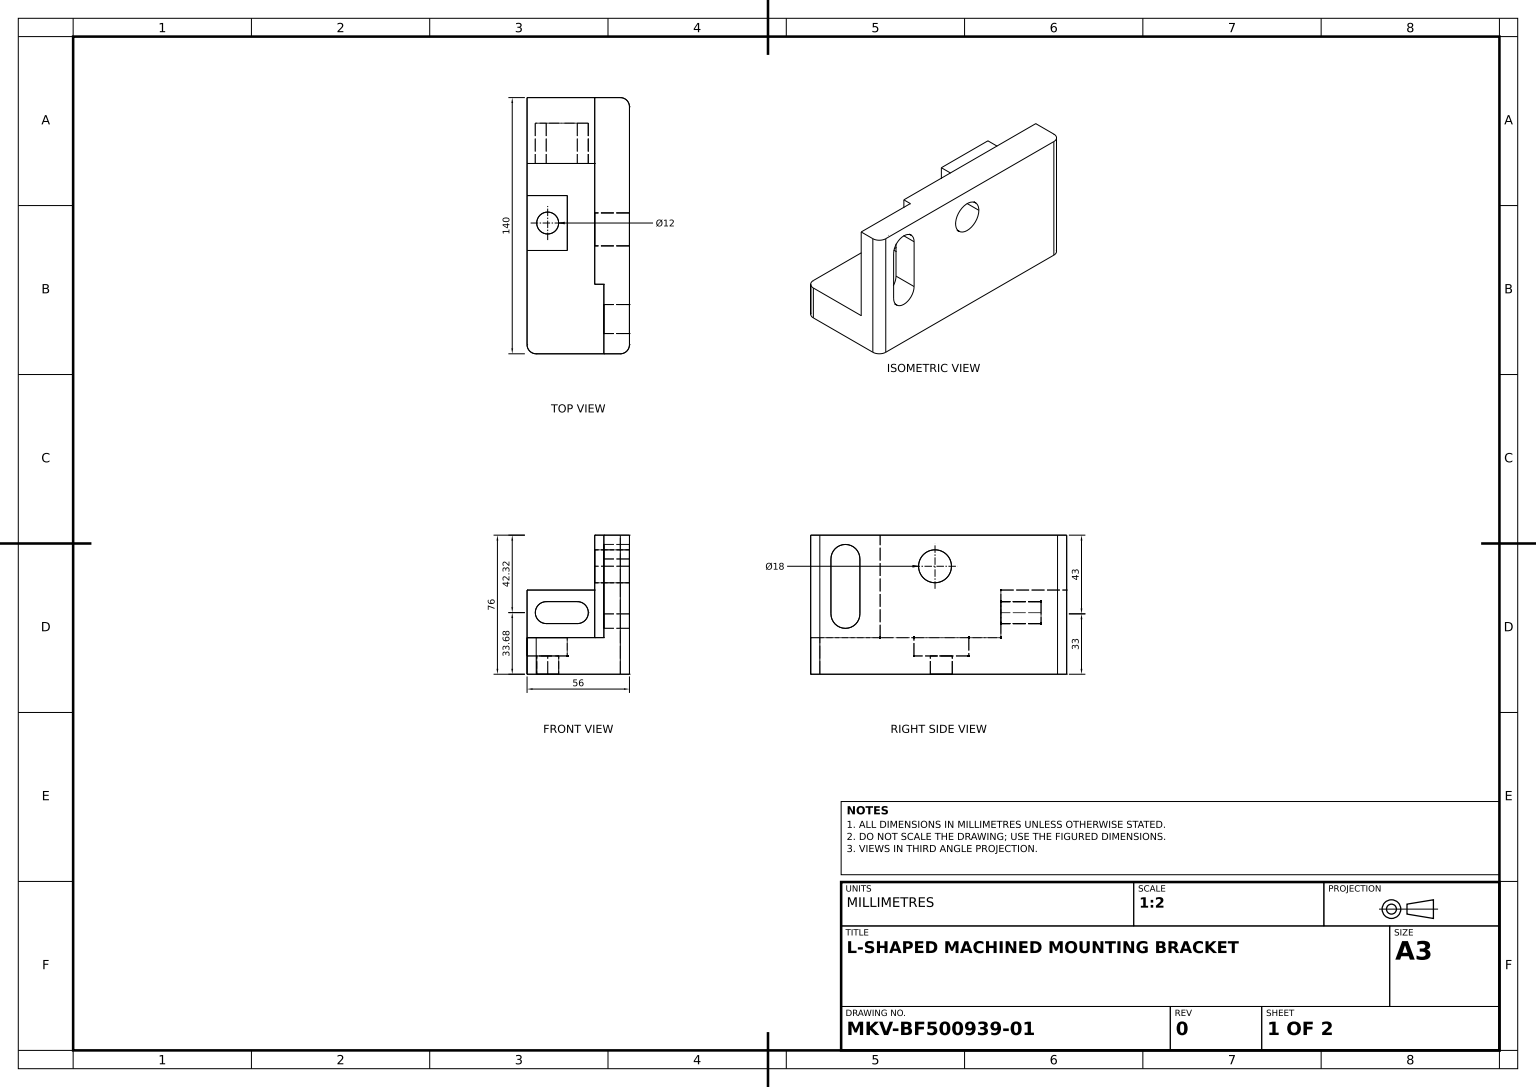
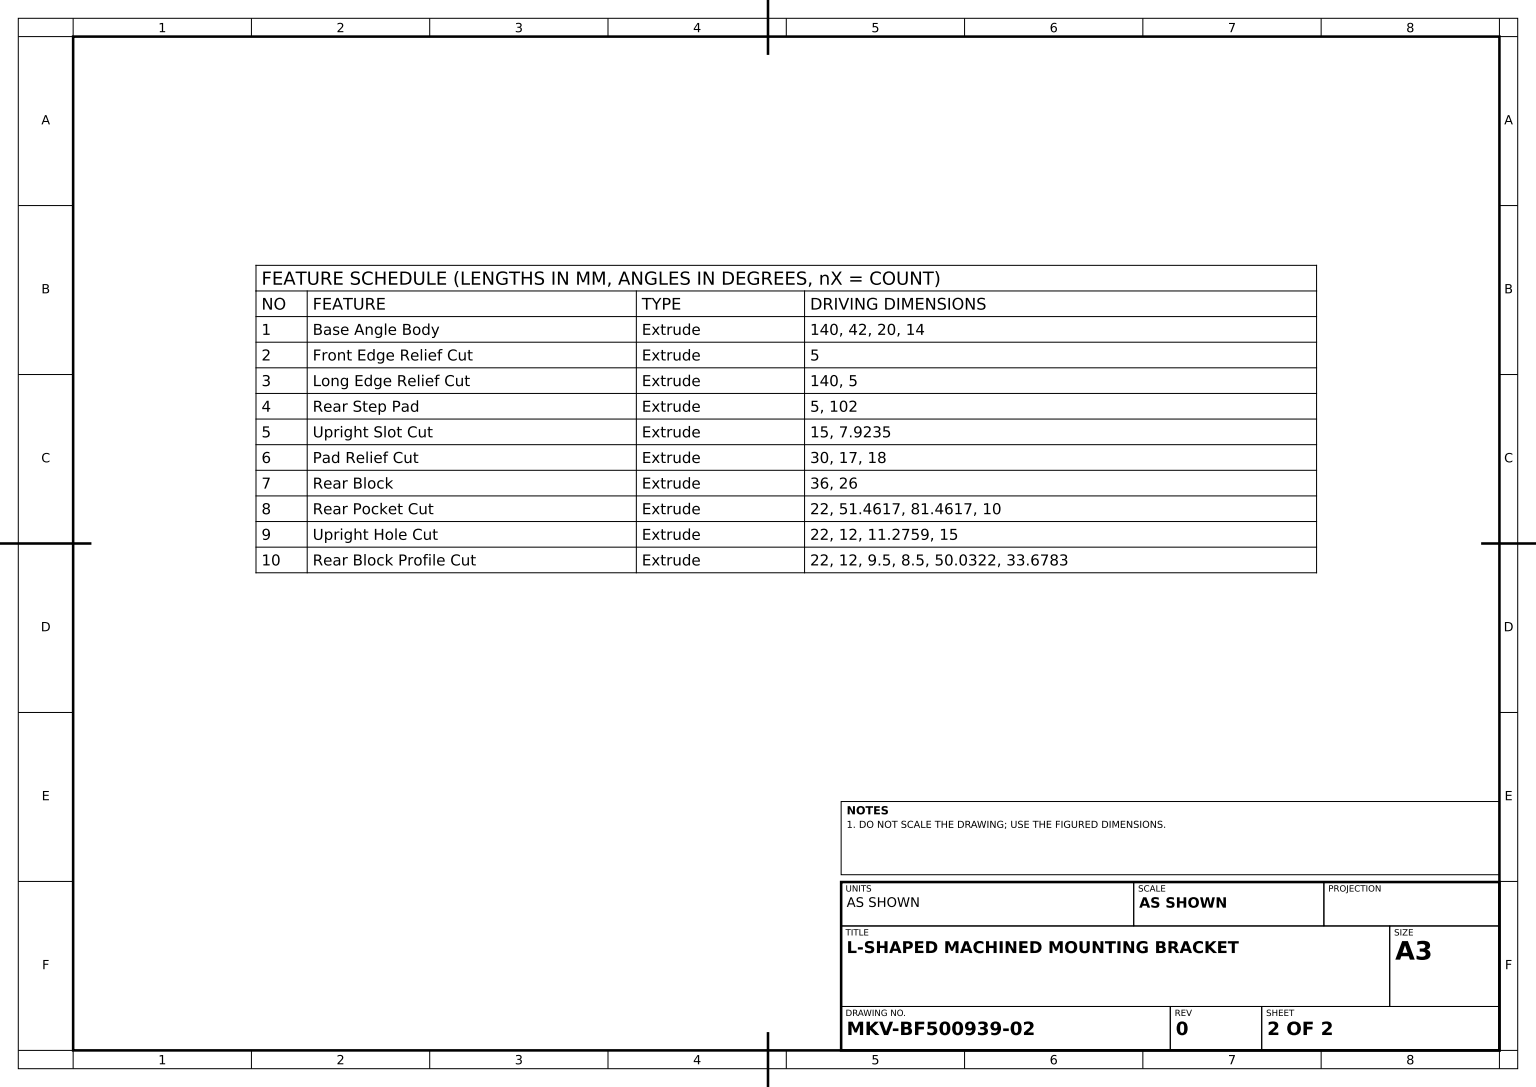
from build123d import *

# Parameters (mm, degrees)
BASE_ANGLE_BODY_DEPTH        = 70
FRONT_EDGE_RELIEF_CUT_DEPTH  = 118.524465538
LONG_EDGE_RELIEF_CUT_DEPTH   = 140
REAR_STEP_PAD_SKETCH_W       = 102
REAR_STEP_PAD_SKETCH_H       = 56
REAR_STEP_PAD_DEPTH          = 5
UPRIGHT_SLOT_CUT_DEPTH       = 112.534747949
PAD_RELIEF_SKETCH_R          = 9
PAD_RELIEF_CUT_DEPTH         = 110.749715262
REAR_BLOCK_SKETCH_W          = 37
REAR_BLOCK_SKETCH_H          = 26
REAR_BLOCK_DEPTH             = 36
REAR_POCKET_SKETCH_W         = 30
REAR_POCKET_SKETCH_H         = 10
REAR_POCKET_CUT_DEPTH        = 22
UPRIGHT_HOLE_SKETCH_R        = 6
UPRIGHT_HOLE_CUT_DEPTH       = 22
REAR_BLOCK_PROFILE_CUT_DEPTH = 22


with BuildPart() as part:
    # Base Angle Profile Sketch → Base Angle Body (new, symmetric)
    with BuildSketch(Plane.XY):
        Polygon((0, 0), (-56, 0), (-56, 20), (-14, 20), (-14, 76), (0, 76), align=None)
    extrude(amount=BASE_ANGLE_BODY_DEPTH, both=True)

    # Front Edge Relief Sketch → Front Edge Relief Cut (cut, through all)
    with BuildSketch(Plane(origin=(0, 76, 0), x_dir=(1, 0, 0), z_dir=(0, 1, 0))):
        with BuildLine():
            Line((-5, 70), (0, 70))
            Line((0, 70), (0, 65))
            ThreePointArc((0, 65), (-1.464466094, 68.535533906), (-5, 70))
        make_face()
        with BuildLine():
            Line((0, -70), (0, -65))
            ThreePointArc((0, -65), (-1.464466094, -68.535533906), (-5, -70))
            Line((-5, -70), (0, -70))
        make_face()
    extrude(amount=-FRONT_EDGE_RELIEF_CUT_DEPTH, mode=Mode.SUBTRACT)

    # Long Edge Relief Sketch → Long Edge Relief Cut (cut)
    with BuildSketch(Plane(origin=(0, 20, 0), x_dir=(1, 0, 0), z_dir=(0, 1, 0))):
        with BuildLine():
            Line((-56, -65), (-56, -70))
            Line((-56, -70), (-51, -70))
            ThreePointArc((-51, -70), (-54.535533906, -68.535533906), (-56, -65))
        make_face()
    extrude(amount=-LONG_EDGE_RELIEF_CUT_DEPTH, mode=Mode.SUBTRACT)

    # Rear Step Pad Sketch → Rear Step Pad (add)
    with BuildSketch(Plane.ZY.offset(14)):
        with Locations((-19, 48)):
            Rectangle(REAR_STEP_PAD_SKETCH_W, REAR_STEP_PAD_SKETCH_H)
    extrude(amount=REAR_STEP_PAD_DEPTH)

    # Upright Slot Sketch → Upright Slot Cut (cut, through all)
    with BuildSketch(Plane.ZY.offset(14)):
        with BuildLine():
            Line((43.076503739, 33), (43.076503739, 63))
            ThreePointArc((43.076503739, 63), (51, 70.923496261), (58.923496261, 63))
            Line((58.923496261, 63), (58.923496261, 33))
            ThreePointArc((58.923496261, 33), (51, 25.076503739), (43.076503739, 33))
        make_face()
    extrude(amount=-UPRIGHT_SLOT_CUT_DEPTH, mode=Mode.SUBTRACT)

    # Pad Relief Sketch → Pad Relief Cut (cut, through all)
    with BuildSketch(Plane.ZY.offset(19)):
        with Locations((2, 59)):
            Circle(PAD_RELIEF_SKETCH_R)
    extrude(amount=-PAD_RELIEF_CUT_DEPTH, mode=Mode.SUBTRACT)

    # Rear Block Sketch → Rear Block (add)
    with BuildSketch(Plane(origin=(0, 0, -70), x_dir=(-1, 0, 0), z_dir=(0, 0, -1))):
        with Locations((37.5, 33)):
            Rectangle(REAR_BLOCK_SKETCH_W, REAR_BLOCK_SKETCH_H)
    extrude(amount=-REAR_BLOCK_DEPTH)

    # Rear Pocket Sketch → Rear Pocket Cut (cut)
    with BuildSketch(Plane.ZY.offset(56)):
        with Locations((-1.461655613, 15)):
            Rectangle(REAR_POCKET_SKETCH_W, REAR_POCKET_SKETCH_H)
    extrude(amount=-REAR_POCKET_CUT_DEPTH, mode=Mode.SUBTRACT)

    # Upright Hole Sketch → Upright Hole Cut (cut)
    with BuildSketch(Plane(origin=(0, 10, 0), x_dir=(1, 0, 0), z_dir=(0, 1, 0))):
        with Locations(Location((-44.72410092, 1.461655613, 0), (0, 0, 270))):
            Circle(UPRIGHT_HOLE_SKETCH_R)
    extrude(amount=-UPRIGHT_HOLE_CUT_DEPTH, mode=Mode.SUBTRACT)

    # Rear Block Profile Sketch → Rear Block Profile Cut (cut)
    with BuildSketch(Plane.XY.offset(-34)):
        with BuildLine():
            Line((-45.5, 39.678271728), (-28.5, 39.678271728))
            ThreePointArc((-28.5, 39.678271728), (-22.5, 33.678271728), (-28.5, 27.678271728))
            Line((-28.5, 27.678271728), (-45.5, 27.678271728))
            ThreePointArc((-45.5, 27.678271728), (-51.5, 33.678271728), (-45.5, 39.678271728))
        make_face()
    extrude(amount=-REAR_BLOCK_PROFILE_CUT_DEPTH, mode=Mode.SUBTRACT)


solid = part.part
